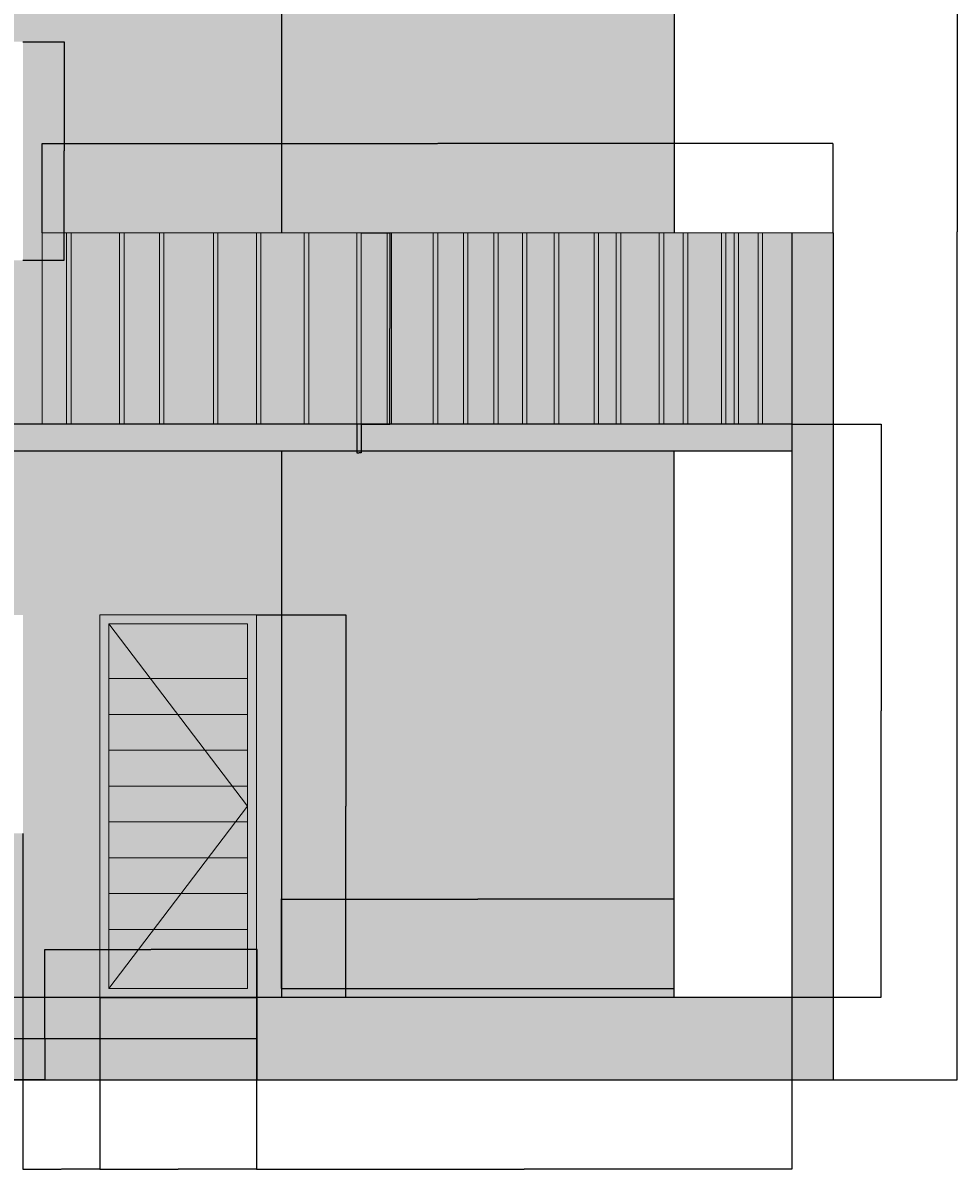
# Model space of a CAD drawing. Units: millimetres. Extents: x 2511 to 24632, y 2213 to 12972.
# Tile 5 of 5: x 19414 to 24632, y 2507 to 8906. Entities that reach past the tile are written whole.
import ezdxf

# ---------------------------------------------------------------- set-up
doc = ezdxf.new("R2010")
doc.units = ezdxf.units.MM
for name, color, linetype, lineweight in [('A-ANNO-DIMS', 2, 'Continuous', 18), ('A-BASE-PATT', 9, 'Continuous', 9), ('A-ELEV', 7, 'Continuous', 25), ('A-ELEV-DOOR', 7, 'Continuous', 18), ('A-ELEV-PATT', 13, 'Continuous', 9), ('A-ELEV-RAIL', 7, 'Continuous', 18), ('A-RAIL-PATT', 7, 'Continuous', 9)]:
    doc.layers.add(name, color=color, linetype=linetype, lineweight=lineweight)
doc.layers.add('A-DOOR-PATT', color=254, linetype='Continuous', lineweight=9, true_color=0xd7ebd2)
doc.styles.get("Standard").update_dxf_attribs({"font": 'arial.ttf'})
doc.dimstyles.get("Standard").update_dxf_attribs({"dimtxt": 0.18, "dimasz": 0.18, "dimexe": 0.18, "dimexo": 0.0625, "dimgap": 0.09, "dimtad": 0, "dimtih": 1, "dimtoh": 1, "dimdec": 4, "dimzin": 0, "dimdsep": 46, "dimtxsty": 'Standard', "dimcen": 0.09, "dimadec": 0, "dimazin": 0, "dimtfac": 1, "dimtdec": 4, "dimtofl": 0, "dimtmove": 0, "dimatfit": 3, "dimfxl": 1, "dimtolj": 1, "dimtzin": 0, "dimarcsym": 0})

# ---------------------------------------------------------------- blocks, each defined once
blk = doc.blocks.new('BALCONY-BALUSTER-25')
blk.add_lwpolyline([(0.0003487384565233, -0.0004698816292148), (25.00034873845653, -0.0004698816292148), (25.00034873845653, 1066.999530118371), (0.0003487384565233, 1066.999530118371)], close=True)
blk = doc.blocks.new('*D15')
at = {"layer": 'A-ANNO-DIMS', "color": 0, "lineweight": -2, "transparency": 16777216}
for p, q in [((21303.96650820039, 7733.216530118373), (21464.1340082004, 7733.216530118373)), ((21463.9540082004, 7733.036530118373), (21463.9540082004, 7199.899599695455)), ((21463.9540082004, 6666.396530118375), (21463.9540082004, 7199.533460541293)), ((21303.96650820039, 6666.216530118375), (21464.1340082004, 6666.216530118375))]:
    blk.add_line(p, q, dxfattribs=at)
at = {"layer": 'A-ANNO-DIMS', "color": 0, "transparency": 16777216}
for points in [[(21463.9240082004, 7733.036530118373), (21463.9840082004, 7733.036530118373), (21463.9540082004, 7733.216530118373)], [(21463.9240082004, 6666.396530118375), (21463.9840082004, 6666.396530118375), (21463.9540082004, 6666.216530118375)]]:
    blk.add_solid(points, dxfattribs=at)
at = {"layer": 'Defpoints', "color": 0, "transparency": 16777216}
for p in [(21303.90400820039, 7733.216530118373), (21463.9540082004, 7733.216530118373), (21303.90400820039, 6666.216530118375)]:
    blk.add_point(p, dxfattribs=at)
at = {"layer": 'A-ANNO-DIMS', "color": 0, "transparency": 16777216, "insert": (21463.95400820039, 7199.716530118367), "char_height": 0.18, "attachment_point": 5}
blk.add_mtext('\\A1;BALUSTER 1067 TYP.', dxfattribs=at)
blk = doc.blocks.new('*D16')
at = {"layer": 'A-ANNO-DIMS', "color": 0, "lineweight": -2, "transparency": 16777216}
for p, q in [((21278.90400820039, 6666.15403011837), (21278.90400820039, 6505.98653011837)), ((21303.90400820039, 6666.15403011837), (21303.90400820039, 6505.98653011837)), ((21279.08400820039, 6506.16653011837), (21290.87438337092, 6506.16653011837)), ((21303.72400820038, 6506.16653011837), (21291.93363302985, 6506.16653011837))]:
    blk.add_line(p, q, dxfattribs=at)
at = {"layer": 'A-ANNO-DIMS', "color": 0, "transparency": 16777216}
for points in [[(21279.08400820039, 6506.19653011837), (21279.08400820039, 6506.136530118372), (21278.90400820039, 6506.16653011837)], [(21303.72400820038, 6506.19653011837), (21303.72400820038, 6506.136530118372), (21303.90400820039, 6506.16653011837)]]:
    blk.add_solid(points, dxfattribs=at)
at = {"layer": 'Defpoints', "color": 0, "transparency": 16777216}
for p in [(21278.90400820039, 6666.21653011837), (21303.90400820039, 6666.21653011837), (21303.90400820039, 6506.16653011837)]:
    blk.add_point(p, dxfattribs=at)
at = {"layer": 'A-ANNO-DIMS', "color": 0, "transparency": 16777216, "insert": (21291.40400820038, 6506.16653011837), "char_height": 0.18, "attachment_point": 5}
blk.add_mtext('\\A1;25 TYP.', dxfattribs=at)
blk = doc.blocks.new('*D34')
at = {"layer": 'A-ANNO-DIMS', "color": 0, "lineweight": -2, "transparency": 16777216}
for p, q in [((19414.05404479581, 8801.216530118374), (19644.59745561891, 8801.216530118374)), ((19644.41745561891, 8801.036530118374), (19644.41745561892, 8191.398433256164)), ((19644.41745561892, 7581.396530118374), (19644.41745561892, 8191.034626980584)), ((19414.05404479581, 7581.216530118374), (19644.59745561892, 7581.216530118374))]:
    blk.add_line(p, q, dxfattribs=at)
at = {"layer": 'A-ANNO-DIMS', "color": 0, "transparency": 16777216}
for points in [[(19644.38745561891, 8801.036530118374), (19644.44745561891, 8801.036530118374), (19644.41745561891, 8801.216530118374)], [(19644.38745561892, 7581.396530118374), (19644.44745561891, 7581.396530118374), (19644.41745561892, 7581.216530118374)]]:
    blk.add_solid(points, dxfattribs=at)
at = {"layer": 'Defpoints', "color": 0, "transparency": 16777216}
for p in [(19413.99154479581, 8801.216530118374), (19644.41745561891, 8801.216530118374), (19413.99154479581, 7581.216530118374)]:
    blk.add_point(p, dxfattribs=at)
at = {"layer": 'A-ANNO-DIMS', "color": 0, "transparency": 16777216, "insert": (19644.41745561891, 8191.216530118365), "char_height": 0.18, "attachment_point": 5}
blk.add_mtext('\\A1;1220 TYP.', dxfattribs=at)
blk = doc.blocks.new('*D65')
at = {"layer": 'A-ANNO-DIMS', "color": 0, "lineweight": -2, "transparency": 16777216}
for p, q in [((21026.52001400001, 12472.75558400001), (24631.73979700003, 12472.75558400001)), ((24631.55979700003, 12472.575584), (24631.55979700003, 7739.667960137794)), ((24631.55979700003, 3006.396530000001), (24631.55979700003, 7739.304153862214)), ((23938.87229700001, 3006.216530000001), (24631.73979700003, 3006.216530000001))]:
    blk.add_line(p, q, dxfattribs=at)
at = {"layer": 'A-ANNO-DIMS', "color": 0, "transparency": 16777216}
for points in [[(24631.52979700003, 12472.575584), (24631.58979700003, 12472.575584), (24631.55979700003, 12472.75558400001)], [(24631.52979700003, 3006.396530000001), (24631.58979700003, 3006.396530000001), (24631.55979700003, 3006.216530000001)]]:
    blk.add_solid(points, dxfattribs=at)
at = {"layer": 'Defpoints', "color": 0, "transparency": 16777216}
for p in [(21026.45751400001, 12472.75558400001), (24631.55979700003, 12472.75558400001), (23938.80979700001, 3006.216530000001)]:
    blk.add_point(p, dxfattribs=at)
at = {"layer": 'A-ANNO-DIMS', "color": 0, "transparency": 16777216, "insert": (24631.55979700002, 7739.486056999995), "char_height": 0.18, "attachment_point": 5}
blk.add_mtext('\\A1;9467', dxfattribs=at)
blk = doc.blocks.new('*D71')
at = {"layer": 'A-ANNO-DIMS', "color": 0, "lineweight": -2, "transparency": 16777216}
for p, q in [((23708.87229700001, 6666.216530000004), (24207.73979700002, 6666.216530000004)), ((24207.55979700002, 6666.036530000003), (24207.55979700002, 5066.398494529334)), ((24207.55979700002, 3466.396530000003), (24207.55979700002, 5066.034565470671)), ((23708.87229700001, 3466.216530000002), (24207.73979700002, 3466.216530000002))]:
    blk.add_line(p, q, dxfattribs=at)
at = {"layer": 'A-ANNO-DIMS', "color": 0, "transparency": 16777216}
for points in [[(24207.52979700002, 6666.036530000003), (24207.58979700002, 6666.036530000003), (24207.55979700002, 6666.216530000004)], [(24207.52979700002, 3466.396530000003), (24207.58979700002, 3466.396530000003), (24207.55979700002, 3466.216530000002)]]:
    blk.add_solid(points, dxfattribs=at)
at = {"layer": 'Defpoints', "color": 0, "transparency": 16777216}
for p in [(23708.80979700001, 6666.216530000004), (23708.80979700001, 3466.216530000002), (24207.55979700002, 3466.216530000002)]:
    blk.add_point(p, dxfattribs=at)
at = {"layer": 'A-ANNO-DIMS', "color": 0, "transparency": 16777216, "insert": (24207.55979700001, 5066.216529999994), "char_height": 0.18, "attachment_point": 5}
blk.add_mtext('\\A1;3200', dxfattribs=at)
blk = doc.blocks.new('*D74')
at = {"layer": 'A-ANNO-DIMS', "color": 0, "lineweight": -2, "transparency": 16777216}
for p, q in [((19413.991545, 4381.15403), (19413.991545, 2507.28653)), ((19843.809797, 3466.154030000001), (19843.809797, 2507.28653)), ((19414.171545, 2507.46653), (19628.50316076808, 2507.46653)), ((19843.629797, 2507.46653), (19629.29818123192, 2507.46653))]:
    blk.add_line(p, q, dxfattribs=at)
at = {"layer": 'A-ANNO-DIMS', "color": 0, "transparency": 16777216}
for points in [[(19414.171545, 2507.49653), (19414.171545, 2507.43653), (19413.991545, 2507.46653)], [(19843.629797, 2507.49653), (19843.629797, 2507.43653), (19843.809797, 2507.46653)]]:
    blk.add_solid(points, dxfattribs=at)
at = {"layer": 'Defpoints', "color": 0, "transparency": 16777216}
for p in [(19413.991545, 4381.216529999999), (19843.809797, 3466.21653), (19843.809797, 2507.46653)]:
    blk.add_point(p, dxfattribs=at)
at = {"layer": 'A-ANNO-DIMS', "color": 0, "transparency": 16777216, "insert": (19628.900671, 2507.46653), "char_height": 0.18, "attachment_point": 5}
blk.add_mtext('\\A1;429.8', dxfattribs=at)
blk = doc.blocks.new('*D75')
at = {"layer": 'A-ANNO-DIMS', "color": 0, "lineweight": -2, "transparency": 16777216}
for p, q in [((19843.809797, 3466.154030000001), (19843.809797, 2507.28653)), ((20718.809797, 3466.154030000001), (20718.809797, 2507.28653)), ((19843.989797, 2507.46653), (20281.02015170669, 2507.46653)), ((20718.629797, 2507.46653), (20281.59944229332, 2507.46653))]:
    blk.add_line(p, q, dxfattribs=at)
at = {"layer": 'A-ANNO-DIMS', "color": 0, "transparency": 16777216}
for points in [[(19843.989797, 2507.49653), (19843.989797, 2507.43653), (19843.809797, 2507.46653)], [(20718.629797, 2507.49653), (20718.629797, 2507.43653), (20718.809797, 2507.46653)]]:
    blk.add_solid(points, dxfattribs=at)
at = {"layer": 'Defpoints', "color": 0, "transparency": 16777216}
for p in [(19843.809797, 3466.21653), (20718.809797, 3466.21653), (20718.809797, 2507.46653)]:
    blk.add_point(p, dxfattribs=at)
at = {"layer": 'A-ANNO-DIMS', "color": 0, "transparency": 16777216, "insert": (20281.309797, 2507.46653), "char_height": 0.18, "attachment_point": 5}
blk.add_mtext('\\A1;875', dxfattribs=at)
blk = doc.blocks.new('*D76')
at = {"layer": 'A-ANNO-DIMS', "color": 0, "lineweight": -2, "transparency": 16777216}
for p, q in [((20718.87229700001, 5601.216530000002), (21217.73979700002, 5601.216530000002)), ((21217.55979700002, 5601.036530000001), (21217.55979700002, 4533.898494529333)), ((21217.55979700002, 3466.396530000003), (21217.55979700002, 4533.534565470669)), ((20718.87229700001, 3466.216530000002), (21217.73979700002, 3466.216530000002))]:
    blk.add_line(p, q, dxfattribs=at)
at = {"layer": 'A-ANNO-DIMS', "color": 0, "transparency": 16777216}
for points in [[(21217.52979700002, 5601.036530000001), (21217.58979700002, 5601.036530000001), (21217.55979700002, 5601.216530000002)], [(21217.52979700002, 3466.396530000003), (21217.58979700002, 3466.396530000003), (21217.55979700002, 3466.216530000002)]]:
    blk.add_solid(points, dxfattribs=at)
at = {"layer": 'Defpoints', "color": 0, "transparency": 16777216}
for p in [(20718.80979700001, 5601.216530000002), (20718.80979700001, 3466.216530000002), (21217.55979700002, 3466.216530000002)]:
    blk.add_point(p, dxfattribs=at)
at = {"layer": 'A-ANNO-DIMS', "color": 0, "transparency": 16777216, "insert": (21217.55979700001, 4533.716529999995), "char_height": 0.18, "attachment_point": 5}
blk.add_mtext('\\A1;2135', dxfattribs=at)
blk = doc.blocks.new('*D77')
at = {"layer": 'A-ANNO-DIMS', "color": 0, "lineweight": -2, "transparency": 16777216}
for p, q in [((20718.809797, 3466.154030000001), (20718.809797, 2507.28653)), ((23708.809797, 3466.154030000001), (23708.809797, 2507.28653)), ((20718.989797, 2507.46653), (22213.449797, 2507.46653)), ((23708.629797, 2507.46653), (22214.169797, 2507.46653))]:
    blk.add_line(p, q, dxfattribs=at)
at = {"layer": 'A-ANNO-DIMS', "color": 0, "transparency": 16777216}
for points in [[(20718.989797, 2507.49653), (20718.989797, 2507.43653), (20718.809797, 2507.46653)], [(23708.629797, 2507.49653), (23708.629797, 2507.43653), (23708.809797, 2507.46653)]]:
    blk.add_solid(points, dxfattribs=at)
at = {"layer": 'Defpoints', "color": 0, "transparency": 16777216}
for p in [(20718.809797, 3466.21653), (23708.809797, 3466.21653), (23708.809797, 2507.46653)]:
    blk.add_point(p, dxfattribs=at)
at = {"layer": 'A-ANNO-DIMS', "color": 0, "transparency": 16777216, "insert": (22213.809797, 2507.46653), "char_height": 0.18, "attachment_point": 5}
blk.add_mtext('\\A1;2990', dxfattribs=at)
blk = doc.blocks.new('*D78')
at = {"layer": 'A-ANNO-DIMS', "color": 0, "lineweight": -2, "transparency": 16777216}
for p, q in [((20858.809797, 3516.279030000001), (20858.809797, 4015.146529999999)), ((20858.989797, 4014.96653), (21954.8478090423, 4014.96653)), ((23051.426435, 4014.96653), (21955.56842295771, 4014.96653)), ((23051.606435, 3516.279030000001), (23051.606435, 4015.146529999999))]:
    blk.add_line(p, q, dxfattribs=at)
at = {"layer": 'A-ANNO-DIMS', "color": 0, "transparency": 16777216}
for points in [[(20858.989797, 4014.99653), (20858.989797, 4014.936529999999), (20858.809797, 4014.96653)], [(23051.426435, 4014.99653), (23051.426435, 4014.936529999999), (23051.606435, 4014.96653)]]:
    blk.add_solid(points, dxfattribs=at)
at = {"layer": 'Defpoints', "color": 0, "transparency": 16777216}
for p in [(23051.606435, 4014.96653), (20858.809797, 3516.216530000001), (23051.606435, 3516.216530000001)]:
    blk.add_point(p, dxfattribs=at)
at = {"layer": 'A-ANNO-DIMS', "color": 0, "transparency": 16777216, "insert": (21955.208116, 4014.96653), "char_height": 0.18, "attachment_point": 5}
blk.add_mtext('\\A1;2193', dxfattribs=at)
blk = doc.blocks.new('*D79')
at = {"layer": 'A-ANNO-DIMS', "color": 0, "lineweight": -2, "transparency": 16777216}
for p, q in [((19536.486833, 3235.134551), (19536.486833, 3734.002051)), ((19536.666833, 3733.822051), (20128.71280745975, 3733.822051)), ((20721.668359, 3733.822051), (20129.62238454024, 3733.822051)), ((20721.848359, 3235.134551), (20721.848359, 3734.002051))]:
    blk.add_line(p, q, dxfattribs=at)
at = {"layer": 'A-ANNO-DIMS', "color": 0, "transparency": 16777216}
for points in [[(19536.666833, 3733.852051), (19536.666833, 3733.792051), (19536.486833, 3733.822051)], [(20721.668359, 3733.852051), (20721.668359, 3733.792051), (20721.848359, 3733.822051)]]:
    blk.add_solid(points, dxfattribs=at)
at = {"layer": 'Defpoints', "color": 0, "transparency": 16777216}
for p in [(20721.848359, 3733.822051), (19536.486833, 3235.072051), (20721.848359, 3235.072051)]:
    blk.add_point(p, dxfattribs=at)
at = {"layer": 'A-ANNO-DIMS', "color": 0, "transparency": 16777216, "insert": (20129.167596, 3733.822051), "char_height": 0.18, "attachment_point": 5}
blk.add_mtext('\\A1;1185.4', dxfattribs=at)
blk = doc.blocks.new('*D80')
at = {"layer": 'A-ANNO-DIMS', "color": 0, "lineweight": -2, "transparency": 16777216}
for p, q in [((19536.424333, 3235.072051000002), (19037.55683300001, 3235.072051000002)), ((19037.73683300001, 3234.892051000001), (19037.73683300001, 3120.826193637791)), ((19037.73683300001, 3006.396530000001), (19037.73683300001, 3120.462387362211)), ((19536.424333, 3006.216530000001), (19037.55683300001, 3006.216530000001))]:
    blk.add_line(p, q, dxfattribs=at)
at = {"layer": 'A-ANNO-DIMS', "color": 0, "transparency": 16777216}
for points in [[(19037.70683300001, 3234.892051000001), (19037.76683300001, 3234.892051000001), (19037.73683300001, 3235.072051000002)], [(19037.70683300001, 3006.396530000001), (19037.76683300001, 3006.396530000001), (19037.73683300001, 3006.216530000001)]]:
    blk.add_solid(points, dxfattribs=at)
at = {"layer": 'Defpoints', "color": 0, "transparency": 16777216}
for p in [(19037.73683300001, 3235.072051000002), (19536.486833, 3235.072051000002), (19536.486833, 3006.216530000001)]:
    blk.add_point(p, dxfattribs=at)
at = {"layer": 'A-ANNO-DIMS', "color": 0, "transparency": 16777216, "insert": (19037.73683300001, 3120.644290499995), "char_height": 0.18, "attachment_point": 5}
blk.add_mtext('\\A1;228.86', dxfattribs=at)
blk = doc.blocks.new('*D81')
at = {"layer": 'A-ANNO-DIMS', "color": 0, "lineweight": -2, "transparency": 16777216}
for p, q in [((19522.169078, 7733.27903), (19522.169078, 8232.146529999998)), ((19522.349078, 8231.96653), (21730.12704322988, 8231.96653)), ((23938.629797, 8231.96653), (21730.85183177013, 8231.96653)), ((23938.809797, 7733.27903), (23938.809797, 8232.146529999998))]:
    blk.add_line(p, q, dxfattribs=at)
at = {"layer": 'A-ANNO-DIMS', "color": 0, "transparency": 16777216}
for points in [[(19522.349078, 8231.99653), (19522.349078, 8231.936529999997), (19522.169078, 8231.96653)], [(23938.629797, 8231.99653), (23938.629797, 8231.936529999997), (23938.809797, 8231.96653)]]:
    blk.add_solid(points, dxfattribs=at)
at = {"layer": 'Defpoints', "color": 0, "transparency": 16777216}
for p in [(23938.809797, 8231.96653), (19522.169078, 7733.216529999999), (23938.809797, 7733.216529999999)]:
    blk.add_point(p, dxfattribs=at)
at = {"layer": 'A-ANNO-DIMS', "color": 0, "transparency": 16777216, "insert": (21730.4894375, 8231.96653), "char_height": 0.18, "attachment_point": 5}
blk.add_mtext('\\A1;4417', dxfattribs=at)

msp = doc.modelspace()

# ---------------------------------------------------------------- hatches: boundary and pattern name
at = {"layer": 'A-BASE-PATT', "transparency": 33554595}
h = msp.add_hatch(color=256, dxfattribs=at)
h.dxf.hatch_style = 1
h.paths.add_polyline_path([(19536.48683262826, 3235.072050511866), (20721.84835936827, 3235.072050511866), (20721.84835936827, 3006.216530118372), (23532.80979657499, 3006.216530118372), (23938.80979657499, 3006.216530118372), (23938.80979657499, 3466.216530118371), (23532.80979657499, 3466.216530118371), (20718.80979657499, 3466.216530118371), (20718.80979657499, 3462.895537400881), (19843.80979657499, 3462.895537400881), (14762.80979657499, 3466.216530118371), (14762.80979657499, 3006.216530118372), (19536.48683262826, 3006.216530118372)])
at = {"layer": 'A-BASE-PATT', "transparency": 33554551}
h = msp.add_hatch(color=256, dxfattribs=at)
h.dxf.hatch_style = 1
h.paths.add_polyline_path([(23051.60643531335, 3516.216530118373), (20858.80979657499, 3516.21653011837), (20858.80979657499, 3466.216530118371), (23051.60643531335, 3466.216530118371)])
at = {"layer": 'A-BASE-PATT', "transparency": 33554595}
h = msp.add_hatch(color=256, dxfattribs=at)
h.dxf.hatch_style = 1
h.paths.add_polyline_path([(20721.84835936827, 3235.072050511866), (19536.48683262826, 3235.072050511866), (19536.48683262826, 3006.216530118372), (20721.84835936827, 3006.216530118372)])
at = {"layer": 'A-DOOR-PATT'}
h = msp.add_hatch(color=256, dxfattribs=at)
h.dxf.hatch_style = 1
h.paths.add_polyline_path([(20718.80979657499, 5601.216530118371), (19843.80979657499, 5601.216530118371), (19843.80979657499, 3466.216530118371), (20718.80979657499, 3466.216530118371)])
h.paths.add_polyline_path([(20668.80979657499, 5551.21653011837), (20668.80979657499, 3516.21653011837), (19893.80979657499, 3516.21653011837), (19893.80979657499, 5551.21653011837)], flags=16)
h = msp.add_hatch(color=256, dxfattribs=at)
h.dxf.hatch_style = 1
h.paths.add_polyline_path([(20668.80979657499, 5551.21653011837), (19893.80979657499, 5551.21653011837), (19893.80979657499, 3516.21653011837), (20668.80979657499, 3516.21653011837)])
at = {"layer": 'A-ELEV-PATT', "transparency": 33554551}
h = msp.add_hatch(color=256, dxfattribs=at)
h.dxf.hatch_style = 1
h.paths.add_polyline_path([(20858.80979657499, 6516.216530118374), (14762.80979657499, 6516.21653011837), (14762.80979657499, 3466.216530118371), (19843.80979657499, 3466.216530118371), (19843.80979657499, 5601.216530118371), (20718.80979657499, 5601.216530118371), (20718.80979657499, 3466.216530118371), (20858.80979657499, 3466.216530118371)])
h.paths.add_polyline_path([(16969.80319715291, 5601.216530118371), (16969.80319715291, 4381.21653011837), (15441.81503455806, 4381.21653011837), (15441.81503455806, 5601.216530118371)], flags=16)
h.paths.add_polyline_path([(16919.80319715291, 5551.21653011837), (16919.80319715291, 4431.21653011837), (15491.81503455806, 4431.21653011837), (15491.81503455806, 5551.21653011837)], flags=0)
h.paths.add_polyline_path([(17877.81880597513, 5601.216530118371), (19413.9915447958, 5601.216530118371), (19413.9915447958, 4381.21653011837), (17886.00338220095, 4381.21653011837), (17877.81880597513, 4381.21653011837)], flags=16)
h.paths.add_polyline_path([(17936.00338220095, 5551.21653011837), (19363.9915447958, 5551.21653011837), (19363.9915447958, 4431.21653011837), (17936.00338220095, 4431.21653011837)], flags=0)
h.paths.add_polyline_path([(20858.80979657499, 9716.216530118376), (14762.80979657499, 9716.21653011837), (14762.80979657499, 6666.21653011837), (19522.169078361, 6666.21653011837), (19522.169078361, 7733.216530118371), (20858.80979657499, 7733.216530118371)])
h.paths.add_polyline_path([(16969.80319715291, 8801.21653011837), (16969.80319715291, 7581.216530118371), (15441.81503455806, 7581.216530118371), (15441.81503455806, 8801.21653011837)], flags=16)
h.paths.add_polyline_path([(16919.80319715291, 8751.216530118369), (16919.80319715291, 7631.216530118371), (15491.81503455806, 7631.216530118371), (15491.81503455806, 8751.216530118369)], flags=0)
h.paths.add_polyline_path([(17877.81880597514, 8801.21653011837), (19413.9915447958, 8801.21653011837), (19413.9915447958, 7581.216530118371), (17886.00338220095, 7581.216530118371), (17877.81880597513, 7581.216530118371)], flags=16)
h.paths.add_polyline_path([(17936.00338220095, 8751.216530118369), (19363.9915447958, 8751.216530118369), (19363.9915447958, 7631.216530118371), (17936.00338220095, 7631.216530118371)], flags=0)
h.paths.add_polyline_path([(23051.60643531334, 9716.216530118376), (20858.80979657499, 9716.21653011837), (20858.80979657499, 7733.216530118371), (23051.60643531334, 7733.216530118371)])
h.paths.add_polyline_path([(23051.60643531335, 6516.216530118374), (20858.80979657499, 6516.216530118374), (20858.80979657499, 3516.21653011837), (23051.60643531335, 3516.21653011837)])
h = msp.add_hatch(color=256, dxfattribs=at)
h.dxf.hatch_style = 1
h.paths.add_polyline_path([(19657.99934873846, 7733.216530118371), (19522.169078361, 7733.216530118371), (19522.169078361, 6666.21653011837), (19657.99934873846, 6666.21653011837)])
h.paths.add_polyline_path([(19953.80078593035, 7733.216530118371), (19682.99934873845, 7733.216530118371), (19682.99934873845, 6666.21653011837), (19953.80078593035, 6666.21653011837)])
h.paths.add_polyline_path([(20176.13470145547, 7733.216530118371), (19978.80078593035, 7733.216530118371), (19978.80078593035, 6666.21653011837), (20176.13470145547, 6666.21653011837)])
h.paths.add_polyline_path([(20478.506693447, 7733.216530118371), (20201.13470145547, 7733.216530118371), (20201.13470145547, 6666.21653011837), (20478.506693447, 6666.21653011837)])
h.paths.add_polyline_path([(20718.62643954274, 7733.216530118371), (20503.506693447, 7733.216530118371), (20503.506693447, 6666.21653011837), (20718.62643954274, 6666.21653011837)])
h.paths.add_polyline_path([(20985.42493149404, 7733.216530118371), (20743.62643954274, 7733.216530118371), (20743.62643954274, 6666.21653011837), (20985.42493149404, 6666.21653011837)])
h.paths.add_polyline_path([(21278.90400820039, 7733.216530118371), (21010.42493149404, 7733.216530118371), (21010.42493149404, 6666.21653011837), (21278.90400820039, 6666.21653011837)])
h.paths.add_polyline_path([(21447.87675421615, 7733.216530118371), (21303.90400820039, 7733.216530118371), (21303.90400820039, 6666.21653011837), (21447.87675421615, 6666.21653011837)])
h.paths.add_polyline_path([(21705.78233088226, 7733.216530118371), (21472.87675421615, 7733.216530118371), (21472.87675421615, 6666.21653011837), (21705.78233088226, 6666.21653011837)])
h.paths.add_polyline_path([(21874.75507689802, 7733.216530118371), (21730.78233088226, 7733.216530118371), (21730.78233088226, 6666.21653011837), (21874.75507689802, 6666.21653011837)])
h.paths.add_polyline_path([(22043.72782291378, 7733.216530118371), (21899.75507689802, 7733.216530118371), (21899.75507689802, 6666.21653011837), (22043.72782291378, 6666.21653011837)])
h.paths.add_polyline_path([(22203.80765364411, 7733.216530118371), (22068.72782291378, 7733.216530118371), (22068.72782291378, 6666.21653011837), (22203.80765364411, 6666.21653011837)])
h.paths.add_polyline_path([(22381.67515384405, 7733.216530118371), (22228.80765364412, 7733.216530118371), (22228.80765364412, 6666.21653011837), (22381.67515384405, 6666.21653011837)])
h.paths.add_polyline_path([(22604.00723047041, 7733.216530118371), (22406.67515384405, 7733.216530118371), (22406.67515384405, 6666.21653011837), (22604.00723047041, 6666.21653011837)])
h.paths.add_polyline_path([(22728.51356116076, 7733.216530118371), (22629.00723047041, 7733.216530118371), (22629.00723047041, 6666.21653011837), (22728.51356116076, 6666.21653011837)])
h.paths.add_polyline_path([(22968.6333072565, 7733.216530118371), (22753.51356116076, 7733.216530118371), (22753.51356116076, 6666.21653011837), (22968.6333072565, 6666.21653011837)])
h.paths.add_polyline_path([(23102.03255323227, 7733.216530118371), (22993.6333072565, 7733.216530118371), (22993.6333072565, 6666.21653011837), (23102.03255323227, 6666.21653011837)])
h.paths.add_polyline_path([(23315.47171457321, 7733.216530118371), (23127.03255323227, 7733.216530118371), (23127.03255323227, 6666.21653011837), (23315.47171457321, 6666.21653011837)])
h.paths.add_polyline_path([(23520.01796062896, 7733.216530118371), (23411.61871465318, 7733.216530118371), (23411.61871465318, 6666.21653011837), (23520.01796062896, 6666.21653011837)])
h.paths.add_polyline_path([(23708.80979657499, 7733.216530118371), (23545.01796062896, 7733.216530118371), (23545.01796062896, 6666.21653011837), (23708.80979657499, 6666.21653011837)])
h = msp.add_hatch(color=256, dxfattribs=at)
h.dxf.hatch_style = 1
h.paths.add_polyline_path([(23386.61871465318, 7733.216530118371), (23340.47171457321, 7733.216530118371), (23340.47171457321, 6666.21653011837), (23386.61871465318, 6666.21653011837)])
h = msp.add_hatch(color=256, dxfattribs=at)
h.dxf.hatch_style = 1
h.paths.add_polyline_path([(23938.80979657499, 7733.216530118371), (23708.80979657499, 7733.216530118371), (23708.80979657499, 3466.216530118371), (23938.80979657499, 3466.216530118371)])
h = msp.add_hatch(color=256, dxfattribs=at)
h.dxf.hatch_style = 1
h.paths.add_polyline_path([(23708.80979657499, 6666.21653011837), (14762.80979657499, 6666.21653011837), (14762.80979657499, 6516.21653011837), (23708.80979657499, 6516.216530118374)])
at = {"layer": 'A-RAIL-PATT', "transparency": 33554551}
h = msp.add_hatch(color=256, dxfattribs=at)
h.dxf.hatch_style = 1
h.paths.add_polyline_path([(19682.99934873845, 7733.216530118371), (19657.99934873846, 7733.216530118371), (19657.99934873846, 6666.21653011837), (19682.99934873845, 6666.21653011837)])
h.paths.add_polyline_path([(19978.80078593035, 7733.216530118371), (19953.80078593035, 7733.216530118371), (19953.80078593035, 6666.21653011837), (19978.80078593035, 6666.21653011837)])
h.paths.add_polyline_path([(20201.13470145547, 7733.216530118371), (20176.13470145547, 7733.216530118371), (20176.13470145547, 6666.21653011837), (20201.13470145547, 6666.21653011837)])
h.paths.add_polyline_path([(20503.506693447, 7733.216530118371), (20478.506693447, 7733.216530118371), (20478.506693447, 6666.21653011837), (20503.506693447, 6666.21653011837)])
h.paths.add_polyline_path([(20743.62643954274, 7733.216530118371), (20718.62643954274, 7733.216530118371), (20718.62643954274, 6666.21653011837), (20743.62643954274, 6666.21653011837)])
h.paths.add_polyline_path([(21010.42493149404, 7733.216530118371), (20985.42493149404, 7733.216530118371), (20985.42493149404, 6666.21653011837), (21010.42493149404, 6666.21653011837)])
h.paths.add_polyline_path([(21303.90400820039, 7733.216530118371), (21278.90400820039, 7733.216530118371), (21278.90400820039, 6666.21653011837), (21303.90400820039, 6666.21653011837)])
h.paths.add_polyline_path([(21472.87675421615, 7733.216530118371), (21447.87675421615, 7733.216530118371), (21447.87675421615, 6666.21653011837), (21472.87675421615, 6666.21653011837)])
h.paths.add_polyline_path([(21730.78233088226, 7733.216530118371), (21705.78233088226, 7733.216530118371), (21705.78233088226, 6666.21653011837), (21730.78233088226, 6666.21653011837)])
h.paths.add_polyline_path([(21899.75507689802, 7733.216530118371), (21874.75507689802, 7733.216530118371), (21874.75507689802, 6666.21653011837), (21899.75507689802, 6666.21653011837)])
h.paths.add_polyline_path([(22068.72782291378, 7733.216530118371), (22043.72782291378, 7733.216530118371), (22043.72782291378, 6666.21653011837), (22068.72782291378, 6666.21653011837)])
h.paths.add_polyline_path([(22228.80765364412, 7733.216530118371), (22203.80765364411, 7733.216530118371), (22203.80765364411, 6666.21653011837), (22228.80765364412, 6666.21653011837)])
h.paths.add_polyline_path([(22406.67515384405, 7733.216530118371), (22381.67515384405, 7733.216530118371), (22381.67515384405, 6666.21653011837), (22406.67515384405, 6666.21653011837)])
h.paths.add_polyline_path([(22629.00723047041, 7733.216530118371), (22604.00723047041, 7733.216530118371), (22604.00723047041, 6666.21653011837), (22629.00723047041, 6666.21653011837)])
h.paths.add_polyline_path([(22753.51356116076, 7733.216530118371), (22728.51356116076, 7733.216530118371), (22728.51356116076, 6666.21653011837), (22753.51356116076, 6666.21653011837)])
h.paths.add_polyline_path([(22993.6333072565, 7733.216530118371), (22968.6333072565, 7733.216530118371), (22968.6333072565, 6666.21653011837), (22993.6333072565, 6666.21653011837)])
h = msp.add_hatch(color=256, dxfattribs=at)
h.dxf.hatch_style = 1
h.paths.add_polyline_path([(23127.03255323227, 7733.216530118371), (23102.03255323227, 7733.216530118371), (23102.03255323227, 6666.21653011837), (23127.03255323227, 6666.21653011837)])
h.paths.add_polyline_path([(23340.47171457321, 7733.216530118371), (23315.47171457321, 7733.216530118371), (23315.47171457321, 6666.21653011837), (23340.47171457321, 6666.21653011837)])
h.paths.add_polyline_path([(23411.61871465318, 7733.216530118371), (23386.61871465318, 7733.216530118371), (23386.61871465318, 6666.21653011837), (23411.61871465318, 6666.21653011837)])
h.paths.add_polyline_path([(23545.01796062896, 7733.216530118371), (23520.01796062896, 7733.216530118371), (23520.01796062896, 6666.21653011837), (23545.01796062896, 6666.21653011837)])

# ---------------------------------------------------------------- linework, layer by layer
at = {"layer": 'A-ELEV'}
for p, q in [((20858.80979657499, 9716.21653011837), (20858.80979657499, 7733.216530118371)), ((23051.60643531334, 9716.216530118376), (23051.60643531334, 7733.216530118371)), ((23708.80979657499, 7733.216530118371), (23708.80979657499, 3466.216530118371)), ((23938.80979657499, 7733.216530118371), (23938.80979657499, 3466.216530118371)), ((23708.80979657499, 6666.21653011837), (14762.80979657499, 6666.21653011837)), ((14762.80979657499, 6516.21653011837), (23708.80979657499, 6516.216530118374)), ((20858.80979657499, 6516.21653011837), (20858.80979657499, 3466.216530118371)), ((23051.60643531335, 3466.216530118373), (23051.60643531335, 6516.216530118374)), ((14762.80979657499, 3466.216530118371), (23532.80979657499, 3466.216530118371)), ((20858.80979657499, 3516.21653011837), (23051.60643531335, 3516.216530118373)), ((23532.80979657499, 3466.216530118371), (23938.80979657499, 3466.216530118371)), ((23938.80979657499, 3466.216530118371), (23938.80979657499, 3006.216530118371)), ((14762.80979657499, 3006.216530118372), (23532.80979657499, 3006.216530118372)), ((23532.80979657499, 3006.216530118372), (23938.80979657499, 3006.216530118372))]:
    msp.add_line(p, q, dxfattribs=at)
msp.add_lwpolyline([(19536.48683262826, 3006.216530118372), (20721.84835936827, 3006.216530118372), (20721.84835936827, 3235.072050511866), (19536.48683262826, 3235.072050511866)], close=True, dxfattribs=at)
at = {"layer": 'A-ELEV-DOOR'}
for p, q in [((19843.80979657499, 3466.216530118373), (19843.80979657499, 5601.216530118371)), ((19843.80979657499, 5601.216530118371), (20718.80979657499, 5601.216530118371)), ((19843.80979657499, 3466.216530118371), (19843.80979657499, 5601.216530118371)), ((19843.80979657499, 5601.216530118371), (20718.80979657499, 5601.216530118371)), ((20718.80979657499, 5601.216530118371), (20718.80979657499, 3466.216530118371)), ((20718.80979657499, 5601.216530118371), (20718.80979657499, 3462.895537400881)), ((19893.80979657499, 5551.21653011837), (20668.80979657499, 4533.71653011837)), ((19893.80979657499, 5245.649548501387), (20668.80979657499, 5245.649548501387)), ((19893.80979657499, 5045.649548501387), (20668.80979657499, 5045.649548501387)), ((19893.80979657499, 4845.649548501388), (20668.80979657499, 4845.649548501388)), ((19893.80979657499, 4645.649548501388), (20668.80979657499, 4645.649548501388)), ((20668.80979657499, 4533.71653011837), (19893.80979657499, 3516.21653011837)), ((19893.80979657499, 4445.649548501387), (20668.80979657499, 4445.649548501387)), ((19893.80979657499, 4245.649548501387), (20668.80979657499, 4245.649548501387)), ((19893.80979657499, 4045.649548501387), (20668.80979657499, 4045.649548501387)), ((19893.80979657499, 3845.649548501388), (20668.80979657499, 3845.649548501388)), ((19843.80979657499, 3466.216530118371), (20718.80979657499, 3466.216530118371)), ((20718.80979657499, 3462.895537400881), (19843.80979657499, 3462.895537400881))]:
    msp.add_line(p, q, dxfattribs=at)
for points in [[(19843.80979657499, 3466.216530118371), (20718.80979657499, 3466.216530118371), (20718.80979657499, 5601.216530118371), (19843.80979657499, 5601.216530118371)], [(19893.80979657499, 3516.21653011837), (20668.80979657499, 3516.21653011837), (20668.80979657499, 5551.21653011837), (19893.80979657499, 5551.21653011837)]]:
    msp.add_lwpolyline(points, close=True, dxfattribs=at)
at = {"layer": 'A-ELEV-RAIL'}
for q in [(23938.80979657499, 7733.216530118371), (23938.80979657499, 7733.216530118371), (19522.169078361, 6666.21653011837)]:
    msp.add_line((19522.169078361, 7733.216530118371), q, dxfattribs=at)

# ---------------------------------------------------------------- block references
for p in [(19657.999, 6666.217), (19657.999, 6666.217), (19953.8004371919, 6666.217), (20176.13435271702, 6666.217), (20478.50634470854, 6666.217), (20718.62609080428, 6666.217), (20985.42458275558, 6666.217), (21278.90365946193, 6666.217), (21447.87640547769, 6666.217), (21705.7819821438, 6666.217), (21874.75472815957, 6666.217), (22043.72747417532, 6666.217), (22203.80730490566, 6666.217), (22381.6748051056, 6666.217), (22604.00688173195, 6666.217), (22728.51321242231, 6666.217), (22968.63295851804, 6666.217), (23102.03220449381, 6666.217), (23315.47136583476, 6666.217), (23386.61836591473, 6666.217), (23520.0176118905, 6666.217)]:
    msp.add_blockref('BALCONY-BALUSTER-25', p, dxfattribs=at)

# ---------------------------------------------------------------- dimensions: what is measured, and where the dimension line sits
at = {"layer": 'A-ANNO-DIMS'}
for base, p1, p2, angle, override, picture, middle in [((24631.55979700003, 12472.75558400001), (23938.809797, 3006.21653), (21026.457514, 12472.755584), 90, {"dimdec": 0, "dimlfac": 1, "dimrnd": 0, "dimzin": 0, "dimdsep": 46, "dimlunit": 2}, '*D65', (24631.55979700002, 7739.486056999995)), ((24207.55979700002, 3466.216530000002), (23708.809797, 6666.216529999999), (23708.809797, 3466.21653), 270, {"dimdec": 0, "dimlfac": 1, "dimrnd": 0, "dimzin": 0, "dimdsep": 46, "dimlunit": 2}, '*D71', (24207.55979700001, 5066.216529999994)), ((21217.55979700002, 3466.216530000002), (20718.809797, 5601.21653), (20718.809797, 3466.21653), 270, {"dimdec": 0, "dimlfac": 1, "dimrnd": 0, "dimzin": 0, "dimdsep": 46, "dimlunit": 2}, '*D76', (21217.55979700001, 4533.716529999995)), ((23051.606435, 4014.96653), (20858.809797, 3516.216530000001), (23051.606435, 3516.216530000001), 8.32e-14, {"dimdec": 0, "dimlfac": 1, "dimrnd": 0, "dimzin": 0, "dimdsep": 46, "dimlunit": 2}, '*D78', (21955.208116, 4014.96653)), ((19037.73683300001, 3235.072051000002), (19536.486833, 3006.21653), (19536.486833, 3235.072051), 90, {"dimdec": 2, "dimlfac": 1, "dimrnd": 0, "dimzin": 0, "dimdsep": 46, "dimlunit": 2}, '*D80', (19037.73683300001, 3120.644290499995))]:
    dim = msp.add_linear_dim(base=base, p1=p1, p2=p2, angle=angle, dimstyle='Standard', override=override, dxfattribs=at)
    dim.commit()
    dim.dimension.update_dxf_attribs({"geometry": picture, "text_midpoint": middle})
for base, p1, p2, text, picture, middle in [((19644.41745561891, 8801.216530118374), (19413.9915447958, 7581.21653011837), (19413.9915447958, 8801.21653011837), '<> TYP.', '*D34', (19644.41745561891, 8191.216530118365)), ((21463.9540082004, 7733.216530118373), (21303.90400820039, 6666.21653011837), (21303.90400820039, 7733.216530118371), 'BALUSTER <> TYP.', '*D15', (21463.95400820039, 7199.716530118367))]:
    dim = msp.add_linear_dim(base=base, p1=p1, p2=p2, angle=90, text=text, dimstyle='Standard', override={"dimdec": 0, "dimlfac": 1, "dimrnd": 0, "dimzin": 0, "dimdsep": 46, "dimlunit": 2}, dxfattribs=at)
    dim.commit()
    dim.dimension.update_dxf_attribs({"geometry": picture, "text_midpoint": middle})
for base, p1, p2, override, picture, middle in [((23938.809797, 8231.96653), (19522.169078, 7733.216529999999), (23938.809797, 7733.216529999999), {"dimdec": 0, "dimlfac": 1, "dimrnd": 0, "dimzin": 0, "dimdsep": 46, "dimlunit": 2}, '*D81', (21730.4894375, 8231.96653)), ((19843.809797, 2507.46653), (19413.991545, 4381.216529999999), (19843.809797, 3466.21653), {"dimdec": 1, "dimlfac": 1, "dimrnd": 0, "dimzin": 0, "dimdsep": 46, "dimlunit": 2}, '*D74', (19628.900671, 2507.46653)), ((20721.848359, 3733.822051), (19536.486833, 3235.072051), (20721.848359, 3235.072051), {"dimdec": 1, "dimlfac": 1, "dimrnd": 0, "dimzin": 0, "dimdsep": 46, "dimlunit": 2}, '*D79', (20129.167596, 3733.822051)), ((20718.809797, 2507.46653), (19843.809797, 3466.21653), (20718.809797, 3466.21653), {"dimdec": 0, "dimlfac": 1, "dimrnd": 0, "dimzin": 0, "dimdsep": 46, "dimlunit": 2}, '*D75', (20281.309797, 2507.46653)), ((23708.809797, 2507.46653), (20718.809797, 3466.21653), (23708.809797, 3466.21653), {"dimdec": 0, "dimlfac": 1, "dimrnd": 0, "dimzin": 0, "dimdsep": 46, "dimlunit": 2}, '*D77', (22213.809797, 2507.46653))]:
    dim = msp.add_linear_dim(base=base, p1=p1, p2=p2, dimstyle='Standard', override=override, dxfattribs=at)
    dim.commit()
    dim.dimension.update_dxf_attribs({"geometry": picture, "text_midpoint": middle})
dim = msp.add_linear_dim(base=(21303.90400820039, 6506.16653011837), p1=(21278.90400820039, 6666.21653011837), p2=(21303.90400820039, 6666.21653011837), text='<> TYP.', dimstyle='Standard', override={"dimdec": 0, "dimlfac": 1, "dimrnd": 0, "dimzin": 0, "dimdsep": 46, "dimlunit": 2}, dxfattribs=at)
dim.commit()
dim.dimension.update_dxf_attribs({"geometry": '*D16', "text_midpoint": (21291.40400820038, 6506.16653011837)})

doc.saveas('drawing.dxf')
